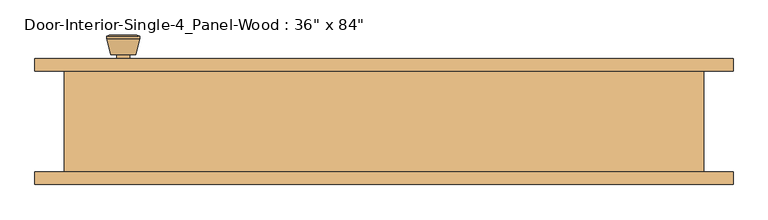
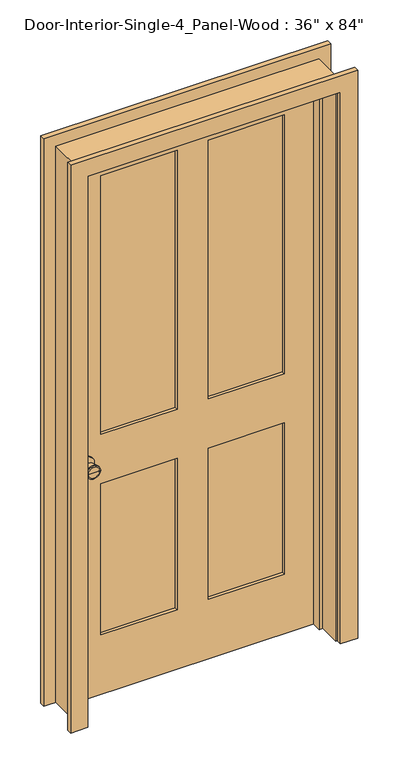
"""IFC4 building model written with IfcOpenShell, lengths in millimetres: door geometry."""

from ifc_helpers import new_model, si_unit, point, frame, frame_2d, origin, place, context, project, spatial, polyline, circle_curve, trimmed, segment, composite_curve, outline, extrude, faceted_brep, source, transform, mapped, element, save
from ifc_brep_helpers import plane_surface, cylinder_surface, revolved_surface, advanced_brep


def door_ecef8289(model_context):
    return source(origin(), model_context, "Body", "SolidModel", [
        advanced_brep(
        [(-393.7, 32.1, 914.4), (-383.7, 32.1, 914.4), (-403.7, 32.1, 914.4), (-373.2241324, -16.9, 914.4), (-393.7, -16.9, 914.4), (-414.1758676, -16.9, 914.4), (-368.7, -15.0721319, 914.4), (-418.7, -15.0721319, 914.4), (-368.7, -11.6084537, 914.4), (-418.7, -11.6084537, 914.4), (-375.063764, 13.1, 914.4), (-412.336236, 13.1, 914.4), (-383.7, 13.1, 914.4), (-403.7, 13.1, 914.4)],
        [
            (0, 1),
            (1, 2, circle_curve(frame((-393.7, 32.1, 914.4), z_axis=(0.0, 1.0, 0.0), x_axis=(-1.0, 0.0, 0.0)), 10.0)),
            (2, 0),
            (2, 1, circle_curve(frame((-393.7, 32.1, 914.4), z_axis=(0.0, 1.0, 0.0), x_axis=(-1.0, 0.0, 0.0)), 10.0)),
            (3, 4),
            (4, 5),
            (5, 3, circle_curve(frame((-393.7, -16.9, 914.4), z_axis=(0.0, -1.0, 0.0), x_axis=(-1.0, 0.0, 0.0)), 20.4758676)),
            (3, 5, circle_curve(frame((-393.7, -16.9, 914.4), z_axis=(0.0, -1.0, 0.0), x_axis=(-1.0, 0.0, 0.0)), 20.4758676)),
            (6, 3),
            (5, 7),
            (7, 6, circle_curve(frame((-393.7, -15.0721319, 914.4), z_axis=(0.0, -1.0, 0.0), x_axis=(-1.0, 0.0, 0.0)), 25.0)),
            (6, 7, circle_curve(frame((-393.7, -15.0721319, 914.4), z_axis=(0.0, -1.0, 0.0), x_axis=(-1.0, 0.0, 0.0)), 25.0)),
            (8, 6),
            (7, 9),
            (9, 8, circle_curve(frame((-393.7, -11.6084537, 914.4), z_axis=(0.0, -1.0, 0.0), x_axis=(-1.0, 0.0, 0.0)), 25.0)),
            (8, 9, circle_curve(frame((-393.7, -11.6084537, 914.4), z_axis=(0.0, -1.0, 0.0), x_axis=(-1.0, 0.0, 0.0)), 25.0)),
            (10, 8),
            (9, 11),
            (11, 10, circle_curve(frame((-393.7, 13.1, 914.4), z_axis=(0.0, -1.0, 0.0), x_axis=(-1.0, 0.0, 0.0)), 18.636236)),
            (10, 11, circle_curve(frame((-393.7, 13.1, 914.4), z_axis=(0.0, -1.0, 0.0), x_axis=(-1.0, 0.0, 0.0)), 18.636236)),
            (12, 10),
            (11, 13),
            (13, 12, circle_curve(frame((-393.7, 13.1, 914.4), z_axis=(0.0, -1.0, 0.0), x_axis=(-1.0, 0.0, 0.0)), 10.0)),
            (12, 13, circle_curve(frame((-393.7, 13.1, 914.4), z_axis=(0.0, -1.0, 0.0), x_axis=(-1.0, 0.0, 0.0)), 10.0)),
            (1, 12),
            (13, 2),
        ],
        [
            plane_surface(frame((-393.7, 32.1, 914.4), z_axis=(0.0, 1.0, 0.0), x_axis=(-1.0, 0.0, 0.0))),
            plane_surface(frame((-393.7, -16.9, 914.4), z_axis=(0.0, -1.0, 0.0), x_axis=(-1.0, 0.0, 0.0))),
            revolved_surface(polyline([(-414.1758676, -16.9, 914.4), (-418.7, -15.0721319, 914.4)]), (-393.7, 32.1, 914.4), (0.0, 1.0, 0.0)),
            cylinder_surface(frame((-393.7, 32.1, 914.4), z_axis=(0.0, 1.0, 0.0), x_axis=(-1.0, 0.0, 0.0)), 25.0),
            revolved_surface(polyline([(-418.7, -11.6084537, 914.4), (-412.336236, 13.1, 914.4)]), (-393.7, 32.1, 914.4), (0.0, 1.0, 0.0)),
            plane_surface(frame((-393.7, 13.1, 914.4), z_axis=(0.0, 1.0, 0.0), x_axis=(-1.0, 0.0, 0.0))),
            cylinder_surface(frame((-393.7, 32.1, 914.4), z_axis=(0.0, 1.0, 0.0), x_axis=(-1.0, 0.0, 0.0)), 10.0),
        ],
        [
            (0, [[1, 2, 3]]),
            (0, [[-3, 4, -1]]),
            (1, [[5, 6, 7]]),
            (1, [[-6, -5, 8]]),
            (2, [[9, -7, 10, 11]]),
            (2, [[-10, -8, -9, 12]]),
            (3, [[13, -11, 14, 15]]),
            (3, [[-14, -12, -13, 16]]),
            (4, [[17, -15, 18, 19]]),
            (4, [[-18, -16, -17, 20]]),
            (5, [[21, -19, 22, 23]]),
            (5, [[-22, -20, -21, 24]]),
            (6, [[25, -23, 26, -2]]),
            (6, [[-26, -24, -25, -4]]),
        ],
    ),
        extrude(outline(composite_curve([segment(trimmed(circle_curve(frame_2d((914.4, -393.7)), 30.0), [point((914.4, -423.7))], [point((914.4, -363.7))], False, "CARTESIAN"), True, "CONTINUOUS"), segment(trimmed(circle_curve(frame_2d((914.4, -393.7)), 30.0), [point((914.4, -363.7))], [point((914.4, -423.7))], False, "CARTESIAN"), True, "CONTINUOUS")], self_intersect=False)), frame((0.0, 32.1, 0.0), z_axis=(0.0, 1.0, 0.0), x_axis=(0.0, 0.0, 1.0)), (0.0, 0.0, 1.0), 6.0),
        advanced_brep(
        [(-393.7, 79.025, 914.4), (-403.7, 79.025, 914.4), (-383.7, 79.025, 914.4), (-373.2241324, 128.025, 914.4), (-414.1758676, 128.025, 914.4), (-393.7, 128.025, 914.4), (-368.7, 126.1971319, 914.4), (-418.7, 126.1971319, 914.4), (-368.7, 122.7334537, 914.4), (-418.7, 122.7334537, 914.4), (-375.063764, 98.025, 914.4), (-412.336236, 98.025, 914.4), (-383.7, 98.025, 914.4), (-403.7, 98.025, 914.4)],
        [
            (0, 1),
            (1, 2, circle_curve(frame((-393.7, 79.025, 914.4), z_axis=(0.0, -1.0, 0.0), x_axis=(-1.0, 0.0, 0.0)), 10.0)),
            (2, 0),
            (2, 1, circle_curve(frame((-393.7, 79.025, 914.4), z_axis=(0.0, -1.0, 0.0), x_axis=(-1.0, 0.0, 0.0)), 10.0)),
            (3, 4, circle_curve(frame((-393.7, 128.025, 914.4), z_axis=(0.0, 1.0, 0.0), x_axis=(-1.0, 0.0, 0.0)), 20.4758676)),
            (4, 5),
            (5, 3),
            (4, 3, circle_curve(frame((-393.7, 128.025, 914.4), z_axis=(0.0, 1.0, 0.0), x_axis=(-1.0, 0.0, 0.0)), 20.4758676)),
            (6, 7, circle_curve(frame((-393.7, 126.1971319, 914.4), z_axis=(0.0, 1.0, 0.0), x_axis=(-1.0, 0.0, 0.0)), 25.0)),
            (7, 4),
            (3, 6),
            (7, 6, circle_curve(frame((-393.7, 126.1971319, 914.4), z_axis=(0.0, 1.0, 0.0), x_axis=(-1.0, 0.0, 0.0)), 25.0)),
            (8, 9, circle_curve(frame((-393.7, 122.7334537, 914.4), z_axis=(0.0, 1.0, 0.0), x_axis=(-1.0, 0.0, 0.0)), 25.0)),
            (9, 7),
            (6, 8),
            (9, 8, circle_curve(frame((-393.7, 122.7334537, 914.4), z_axis=(0.0, 1.0, 0.0), x_axis=(-1.0, 0.0, 0.0)), 25.0)),
            (10, 11, circle_curve(frame((-393.7, 98.025, 914.4), z_axis=(0.0, 1.0, 0.0), x_axis=(-1.0, 0.0, 0.0)), 18.636236)),
            (11, 9),
            (8, 10),
            (11, 10, circle_curve(frame((-393.7, 98.025, 914.4), z_axis=(0.0, 1.0, 0.0), x_axis=(-1.0, 0.0, 0.0)), 18.636236)),
            (12, 13, circle_curve(frame((-393.7, 98.025, 914.4), z_axis=(0.0, 1.0, 0.0), x_axis=(-1.0, 0.0, 0.0)), 10.0)),
            (13, 11),
            (10, 12),
            (13, 12, circle_curve(frame((-393.7, 98.025, 914.4), z_axis=(0.0, 1.0, 0.0), x_axis=(-1.0, 0.0, 0.0)), 10.0)),
            (1, 13),
            (12, 2),
        ],
        [
            plane_surface(frame((-393.7, 79.025, 914.4), z_axis=(0.0, -1.0, 0.0), x_axis=(-1.0, 0.0, 0.0))),
            plane_surface(frame((-393.7, 128.025, 914.4), z_axis=(0.0, 1.0, 0.0), x_axis=(-1.0, 0.0, 0.0))),
            revolved_surface(polyline([(-414.1758676, 128.025, 914.4), (-418.7, 126.1971319, 914.4)]), (-393.7, 79.025, 914.4), (0.0, -1.0, 0.0)),
            cylinder_surface(frame((-393.7, 79.025, 914.4), z_axis=(0.0, -1.0, 0.0), x_axis=(-1.0, 0.0, 0.0)), 25.0),
            revolved_surface(polyline([(-418.7, 122.7334537, 914.4), (-412.336236, 98.025, 914.4)]), (-393.7, 79.025, 914.4), (0.0, -1.0, 0.0)),
            plane_surface(frame((-393.7, 98.025, 914.4), z_axis=(0.0, -1.0, 0.0), x_axis=(-1.0, 0.0, 0.0))),
            cylinder_surface(frame((-393.7, 79.025, 914.4), z_axis=(0.0, -1.0, 0.0), x_axis=(-1.0, 0.0, 0.0)), 10.0),
        ],
        [
            (0, [[1, 2, 3]]),
            (0, [[-3, 4, -1]]),
            (1, [[5, 6, 7]]),
            (1, [[8, -7, -6]]),
            (2, [[9, 10, -5, 11]]),
            (2, [[12, -11, -8, -10]]),
            (3, [[13, 14, -9, 15]]),
            (3, [[16, -15, -12, -14]]),
            (4, [[17, 18, -13, 19]]),
            (4, [[20, -19, -16, -18]]),
            (5, [[21, 22, -17, 23]]),
            (5, [[24, -23, -20, -22]]),
            (6, [[-2, 25, -21, 26]]),
            (6, [[-4, -26, -24, -25]]),
        ],
    ),
        extrude(outline(composite_curve([segment(trimmed(circle_curve(frame_2d((914.4, -393.7)), 30.0), [point((914.4, -423.7))], [point((914.4, -363.7))], False, "CARTESIAN"), True, "CONTINUOUS"), segment(trimmed(circle_curve(frame_2d((914.4, -393.7)), 30.0), [point((914.4, -363.7))], [point((914.4, -423.7))], False, "CARTESIAN"), True, "CONTINUOUS")], self_intersect=False)), frame((0.0, 73.025, 0.0), z_axis=(0.0, 1.0, 0.0), x_axis=(0.0, 0.0, 1.0)), (0.0, 0.0, 1.0), 6.0),
        faceted_brep([(482.6, 73.025, 0.0), (482.6, -79.375, 0.0), (457.2, -79.375, 0.0), (457.2, 3.175, 0.0), (444.5, 3.175, 0.0), (444.5, 38.1, 0.0), (457.2, 38.1, 0.0), (457.2, 73.025, 0.0), (482.6, 73.025, 2159.0), (482.6, -79.375, 2159.0), (-482.6, -79.375, 2159.0), (-482.6, -79.375, 0.0), (-457.2, -79.375, 0.0), (-457.2, -79.375, 2133.6), (457.2, -79.375, 2133.6), (457.2, 3.175, 2133.6), (-457.2, 3.175, 2133.6), (-457.2, 3.175, 0.0), (-444.5, 3.175, 0.0), (-444.5, 3.175, 2120.9), (444.5, 3.175, 2120.9), (444.5, 38.1, 2120.9), (-444.5, 38.1, 2120.9), (-444.5, 38.1, 0.0), (-457.2, 38.1, 0.0), (-457.2, 38.1, 2133.6), (457.2, 38.1, 2133.6), (457.2, 73.025, 2133.6), (-457.2, 73.025, 2133.6), (-457.2, 73.025, 0.0), (-482.6, 73.025, 0.0), (-482.6, 73.025, 2159.0)], [[[0, 1, 2, 3, 4, 5, 6, 7]], [[1, 0, 8, 9]], [[2, 1, 9, 10, 11, 12, 13, 14]], [[3, 2, 14, 15]], [[4, 3, 15, 16, 17, 18, 19, 20]], [[5, 4, 20, 21]], [[6, 5, 21, 22, 23, 24, 25, 26]], [[7, 6, 26, 27]], [[0, 7, 27, 28, 29, 30, 31, 8]], [[9, 8, 31, 10]], [[15, 14, 13, 16]], [[21, 20, 19, 22]], [[27, 26, 25, 28]], [[30, 29, 24, 23, 18, 17, 12, 11]], [[10, 31, 30, 11]], [[16, 13, 12, 17]], [[22, 19, 18, 23]], [[28, 25, 24, 29]]]),
        extrude(outline(polyline([(2133.6, -457.2), (0.0, -457.2), (0.0, 457.2), (2133.6, 457.2), (2133.6, -457.2)]), holes=[polyline([(2014.5375, 57.15), (2014.5375, 336.55), (1009.65, 336.55), (1009.65, 57.15), (2014.5375, 57.15)]), polyline([(1009.65, -57.15), (1009.65, -336.55), (2014.5375, -336.55), (2014.5375, -57.15), (1009.65, -57.15)]), polyline([(819.15, 57.15), (819.15, 336.55), (231.775, 336.55), (231.775, 57.15), (819.15, 57.15)]), polyline([(231.775, -57.15), (231.775, -336.55), (819.15, -336.55), (819.15, -57.15), (231.775, -57.15)])]), frame((0.0, 38.1, 0.0), z_axis=(0.0, 1.0, 0.0), x_axis=(0.0, 0.0, 1.0)), (0.0, 0.0, 1.0), 34.925),
        extrude(outline(polyline([(336.55, 49.7416667), (57.15, 49.7416667), (57.15, 61.3833333), (336.55, 61.3833333), (336.55, 49.7416667)])), frame((0.0, 0.0, 1009.65), z_axis=(0.0, 0.0, 1.0), x_axis=(1.0, 0.0, 0.0)), (0.0, 0.0, 1.0), 1004.8875),
        extrude(outline(polyline([(-57.15, 49.7416667), (-336.55, 49.7416667), (-336.55, 61.3833333), (-57.15, 61.3833333), (-57.15, 49.7416667)])), frame((0.0, 0.0, 1009.65), z_axis=(0.0, 0.0, 1.0), x_axis=(1.0, 0.0, 0.0)), (0.0, 0.0, 1.0), 1004.8875),
        extrude(outline(polyline([(336.55, 49.7416667), (57.15, 49.7416667), (57.15, 61.3833333), (336.55, 61.3833333), (336.55, 49.7416667)])), frame((0.0, 0.0, 231.775), z_axis=(0.0, 0.0, 1.0), x_axis=(1.0, 0.0, 0.0)), (0.0, 0.0, 1.0), 587.375),
        extrude(outline(polyline([(-57.15, 49.7416667), (-336.55, 49.7416667), (-336.55, 61.3833333), (-57.15, 61.3833333), (-57.15, 49.7416667)])), frame((0.0, 0.0, 231.775), z_axis=(0.0, 0.0, 1.0), x_axis=(1.0, 0.0, 0.0)), (0.0, 0.0, 1.0), 587.375),
        extrude(outline(polyline([(0.0, 463.55), (0.0, 527.05), (2203.45, 527.05), (2203.45, -527.05), (0.0, -527.05), (0.0, -463.55), (2139.95, -463.55), (2139.95, 463.55), (0.0, 463.55)])), frame((0.0, 73.025, 0.0), z_axis=(0.0, 1.0, 0.0), x_axis=(0.0, 0.0, 1.0)), (0.0, 0.0, 1.0), 19.05),
        extrude(outline(polyline([(0.0, 463.55), (0.0, 527.05), (2203.45, 527.05), (2203.45, -527.05), (0.0, -527.05), (0.0, -463.55), (2139.95, -463.55), (2139.95, 463.55), (0.0, 463.55)])), frame((0.0, -98.425, 0.0), z_axis=(0.0, 1.0, 0.0), x_axis=(0.0, 0.0, 1.0)), (0.0, 0.0, 1.0), 19.05),
    ])


if __name__ == "__main__":
    model = new_model("IFC4")
    model_context = context("Model", 3, world=origin())
    ifc_project = project(units=[si_unit("LENGTHUNIT", "METRE", prefix="MILLI")], contexts=[model_context])
    site = spatial("IfcSite", under=ifc_project)
    building = spatial("IfcBuilding", under=site)
    placement = place(None, origin())
    door_shape = door_ecef8289(model_context)
    element("IfcDoor", 1, ObjectType="Door-Interior-Single-4_Panel-Wood : 36\" x 84\"", at=placement, inside=building, context=model_context, shape_type="MappedRepresentation", body=[
        mapped(door_shape, transform((0.0, 0.0, 0.0), x_axis=(1.0, 0.0, 0.0), y_axis=(0.0, 1.0, 0.0), z_axis=(0.0, 0.0, 1.0))),
    ])
    save(model, "model.ifc")

# Revit data of these elements
# Type "Door-Interior-Single-4_Panel-Wood : 36\" x 84\""
#   Type Mark = "8"
#   Assembly Code = "C1020300"
#   Analytic Construction = "Wooden"
#   Top Rail = 0' - 4 11/16"
#   Thickness = 0' - 1 3/8"
#   Thermal Resistance (R) = 2.5876 (h·ft²·°F)/BTU
#   Swing Angle [instance default] = 90.00°
#   Stiles = 0' - 4 3/4"
#   Rough Width = 3' - 2"
#   Rough Height = 7' - 1"
#   Mullion = 0' - 4 1/2"
#   Lock Rail = 0' - 7 1/2"
#   Height = 7' - 0"
#   Width = 3' - 0"
#   Heat Transfer Coefficient (U) = 0.3865 BTU/(h·ft²·°F)
#   Bottom Rail = 0' - 9 1/8"
#   Trim Material = Cherry
#   Panel Material = Cherry
#   Frame Material = Cherry
#   Door Handle Material = Aluminum
#   Visual Light Transmittance = 0
#   Solar Heat Gain Coefficient = 0
#   Wall Closure = (empty or 0)
#   Function = (empty or 0)
# Element 1 (IfcDoor, "Door-Interior-Single-4_Panel-Wood : 36\" x 84\"")
#   Materials on its faces: "Cherry", "Aluminum"
# Materials
#   "Cherry": class "Wood", colour RGB 226 177 128, transparency 0, Description = "Prunus Serotina", Cost = 0
#   "Aluminum": class "Metal", colour RGB 247 247 247, transparency 0, Description = "Aluminum 6061", Cost = 0
